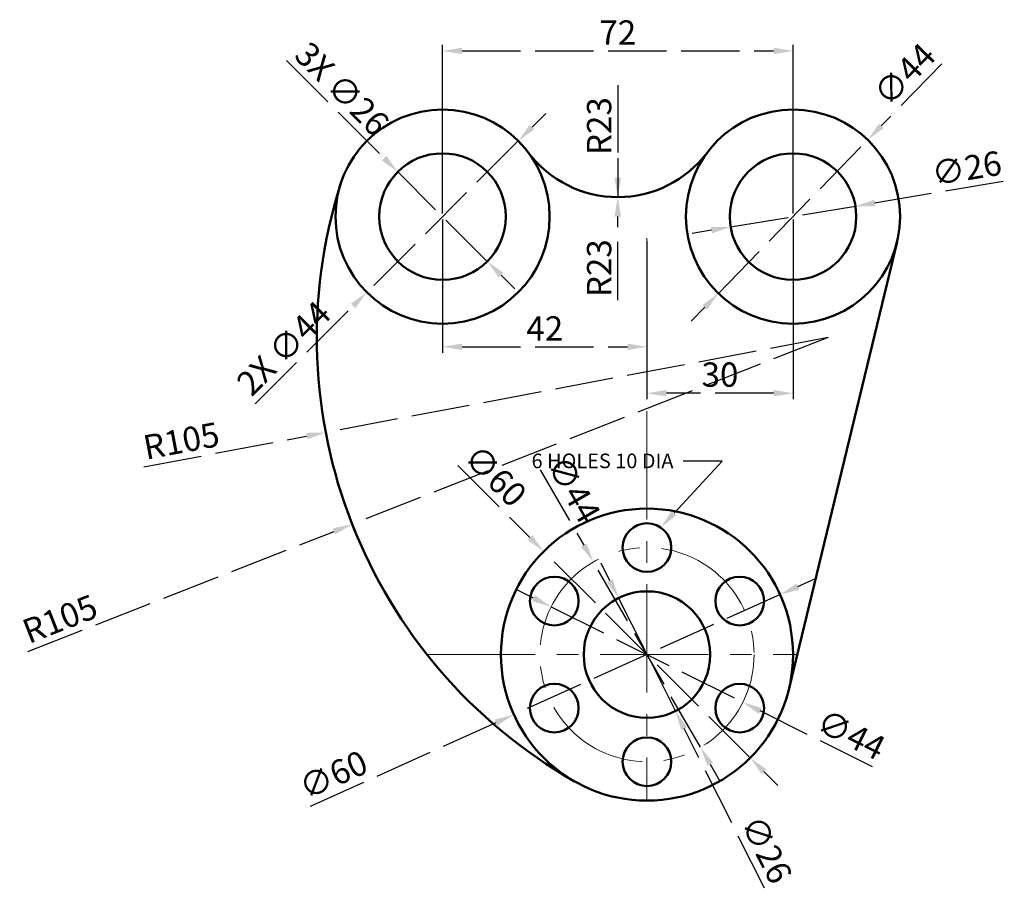
# Model space of a CAD drawing. Units: millimetres. Extents: x 2907 to 3109, y 1232 to 1411.
import ezdxf
from ezdxf import colors
from ezdxf.entities.mleader import LeaderData, LeaderLine
from ezdxf.math import Vec2, Vec3

# ---------------------------------------------------------------- set-up
doc = ezdxf.new("R2010")
doc.units = ezdxf.units.MM
doc.linetypes.add('ACAD_ISO02W100', pattern=[15, 12, -3])
doc.linetypes.add('CENTER', pattern=[50.8, 31.75, -6.35, 6.35, -6.35])
for name, color, linetype, lineweight in [('M-CNTR', 4, 'CENTER', 18), ('M-DIMS', 2, 'Continuous', 25), ('M-OUTL', 7, 'Continuous', 50), ('M-TEXT', 7, 'Continuous', 25)]:
    doc.layers.add(name, color=color, linetype=linetype, lineweight=lineweight)
doc.styles.get("Standard").update_dxf_attribs({"font": 'arial.ttf'})
doc.dimstyles.new('ISO-25', dxfattribs={"dimtxt": 5, "dimasz": 4, "dimexe": 1.25, "dimexo": 0.625, "dimtad": 1, "dimtxsty": 'Standard', "dimcen": 4, "dimadec": 0, "dimazin": 0, "dimtfac": 1, "dimtmove": 0, "dimatfit": 3, "dimfxl": 1, "dimlwd": -1, "dimarcsym": 0})

# ---------------------------------------------------------------- blocks, each defined once
blk = doc.blocks.new('*U1')
blk.add_circle((0, 0), 5)
blk = doc.blocks.new('*U2')
at = {"layer": 'M-OUTL', "color": 0, "linetype": 'ByBlock', "lineweight": -2, "transparency": 16777216}
blk.add_blockref('*U1', (3035.42, 1302.18), dxfattribs=at)
for p, rotation in [((3016.37, 1291.18), 59.99999999999999), ((3054.47, 1291.18), 300), ((3016.37, 1269.18), 120), ((3054.47, 1269.18), 240), ((3035.42, 1258.18), 180)]:
    blk.add_blockref('*U1', p, dxfattribs=dict(at, rotation=rotation))
blk = doc.blocks.new('*D3')
at = {"layer": 'Defpoints', "color": 0, "transparency": 16777216}
for p in [(3065.42, 1404.23), (2993.42, 1370.18), (3065.42, 1370.18)]:
    blk.add_point(p, dxfattribs=at)
at = {"layer": 'M-DIMS', "color": 0, "lineweight": -2, "transparency": 16777216}
for p, q in [((2993.42, 1370.81), (2993.42, 1405.48)), ((3065.42, 1370.81), (3065.42, 1405.48))]:
    blk.add_line(p, q, dxfattribs=at)
at = {"layer": 'M-DIMS', "color": 0, "linetype": 'ACAD_ISO02W100', "transparency": 16777216}
blk.add_line((2997.42, 1404.23), (3061.42, 1404.23), dxfattribs=at)
at = {"layer": 'M-DIMS', "color": 0, "transparency": 16777216}
for points in [[(2997.42, 1404.9), (2997.42, 1403.56), (2993.42, 1404.23)], [(3061.42, 1404.9), (3061.42, 1403.56), (3065.42, 1404.23)]]:
    blk.add_solid(points, dxfattribs=at)
at = {"layer": 'M-DIMS', "color": 0, "transparency": 16777216, "insert": (3029.42, 1407.36), "char_height": 5, "attachment_point": 5}
blk.add_mtext('72', dxfattribs=at)
blk = doc.blocks.new('*D4')
at = {"layer": 'Defpoints', "color": 0, "transparency": 16777216}
for p in [(3072.61, 1345.31), (2969.43, 1325.82)]:
    blk.add_point(p, dxfattribs=at)
at = {"layer": 'M-DIMS', "color": 0, "linetype": 'ACAD_ISO02W100', "transparency": 16777216}
for p, q in [((3072.61, 1345.31), (2969.43, 1325.82)), ((2932.05, 1318.76), (2965.5, 1325.08))]:
    blk.add_line(p, q, dxfattribs=at)
at = {"layer": 'M-DIMS', "color": 0, "transparency": 16777216}
blk.add_solid([(2965.38, 1325.74), (2965.63, 1324.43), (2969.43, 1325.82)], dxfattribs=at)
at = {"layer": 'M-DIMS', "color": 0, "transparency": 16777216, "insert": (2939.87, 1323.48), "char_height": 5, "attachment_point": 5, "rotation": 10.6961}
blk.add_mtext('R105', dxfattribs=at)
blk = doc.blocks.new('*D5')
at = {"layer": 'Defpoints', "color": 0, "transparency": 16777216}
for p in [(3029.42, 1397.18), (3029.42, 1374.18)]:
    blk.add_point(p, dxfattribs=at)
at = {"layer": 'M-DIMS', "color": 0, "linetype": 'ACAD_ISO02W100', "transparency": 16777216}
blk.add_line((3029.42, 1395.38), (3029.42, 1378.18), dxfattribs=at)
at = {"layer": 'M-DIMS', "color": 0, "transparency": 16777216}
blk.add_solid([(3028.75, 1378.18), (3030.09, 1378.18), (3029.42, 1374.18)], dxfattribs=at)
at = {"layer": 'M-DIMS', "color": 0, "transparency": 16777216, "insert": (3026.24, 1388.78), "char_height": 5, "attachment_point": 5, "rotation": 90}
blk.add_mtext('R23', dxfattribs=at)
blk = doc.blocks.new('*D6')
at = {"layer": 'Defpoints', "color": 0, "transparency": 16777216}
for p in [(3062.77, 1292.5), (3008.07, 1267.86)]:
    blk.add_point(p, dxfattribs=at)
at = {"layer": 'M-DIMS', "color": 0, "linetype": 'ACAD_ISO02W100', "transparency": 16777216}
for p, q in [((3066.42, 1294.15), (3070.07, 1295.79)), ((3062.77, 1292.5), (3008.07, 1267.86)), ((2966.29, 1249.04), (3004.42, 1266.22))]:
    blk.add_line(p, q, dxfattribs=at)
at = {"layer": 'M-DIMS', "color": 0, "transparency": 16777216}
for points in [[(3066.15, 1294.76), (3066.69, 1293.54), (3062.77, 1292.5)], [(3004.15, 1266.82), (3004.7, 1265.61), (3008.07, 1267.86)]]:
    blk.add_solid(points, dxfattribs=at)
at = {"layer": 'M-DIMS', "color": 0, "transparency": 16777216, "insert": (2971.24, 1254.9), "char_height": 5, "attachment_point": 5, "rotation": 24.2528}
blk.add_mtext('∅60', dxfattribs=at)
blk = doc.blocks.new('*D7')
at = {"layer": 'Defpoints', "color": 0, "transparency": 16777216}
for p in [(3015.72, 1289.98), (3055.12, 1270.38)]:
    blk.add_point(p, dxfattribs=at)
at = {"layer": 'M-DIMS', "color": 0, "linetype": 'ACAD_ISO02W100', "transparency": 16777216}
for p, q in [((3012.14, 1291.76), (3008.56, 1293.54)), ((3015.72, 1289.98), (3055.12, 1270.38)), ((3081.78, 1257.11), (3058.7, 1268.6))]:
    blk.add_line(p, q, dxfattribs=at)
at = {"layer": 'M-DIMS', "color": 0, "transparency": 16777216}
for points in [[(3012.44, 1292.36), (3011.85, 1291.17), (3015.72, 1289.98)], [(3059, 1269.2), (3058.4, 1268), (3055.12, 1270.38)]]:
    blk.add_solid(points, dxfattribs=at)
at = {"layer": 'M-DIMS', "color": 0, "transparency": 16777216, "insert": (3077.07, 1263.17), "char_height": 5, "attachment_point": 5, "rotation": 333.5478}
blk.add_mtext('∅44', dxfattribs=at)
blk = doc.blocks.new('*D8')
at = {"layer": 'Defpoints', "color": 0, "transparency": 16777216}
for p in [(3029.58, 1291.8), (3041.26, 1268.57)]:
    blk.add_point(p, dxfattribs=at)
at = {"layer": 'M-DIMS', "color": 0, "linetype": 'ACAD_ISO02W100', "transparency": 16777216}
for p, q in [((3027.78, 1295.37), (3025.99, 1298.94)), ((3029.58, 1291.8), (3041.26, 1268.57)), ((3059.56, 1232.18), (3043.06, 1264.99))]:
    blk.add_line(p, q, dxfattribs=at)
at = {"layer": 'M-DIMS', "color": 0, "transparency": 16777216}
for points in [[(3028.38, 1295.67), (3027.19, 1295.07), (3029.58, 1291.8)], [(3043.65, 1265.29), (3042.46, 1264.69), (3041.26, 1268.57)]]:
    blk.add_solid(points, dxfattribs=at)
at = {"layer": 'M-DIMS', "color": 0, "transparency": 16777216, "insert": (3059.41, 1239.85), "char_height": 5, "attachment_point": 5, "rotation": 296.6959}
blk.add_mtext('∅26', dxfattribs=at)
blk = doc.blocks.new('*D9')
at = {"layer": 'Defpoints', "color": 0, "transparency": 16777216}
for p in [(3080.76, 1385.95), (3050.08, 1354.41)]:
    blk.add_point(p, dxfattribs=at)
at = {"layer": 'M-DIMS', "color": 0, "linetype": 'ACAD_ISO02W100', "transparency": 16777216}
for p, q in [((3095.98, 1401.6), (3083.55, 1388.82)), ((3050.08, 1354.41), (3080.76, 1385.95)), ((3047.29, 1351.54), (3044.5, 1348.68))]:
    blk.add_line(p, q, dxfattribs=at)
at = {"layer": 'M-DIMS', "color": 0, "transparency": 16777216}
for points in [[(3083.07, 1389.28), (3084.03, 1388.35), (3080.76, 1385.95)], [(3046.82, 1352.01), (3047.77, 1351.08), (3050.08, 1354.41)]]:
    blk.add_solid(points, dxfattribs=at)
at = {"layer": 'M-DIMS', "color": 0, "transparency": 16777216, "insert": (3088.78, 1398.96), "char_height": 5, "attachment_point": 5, "rotation": 45.7945}
blk.add_mtext('∅44', dxfattribs=at)
blk = doc.blocks.new('*D10')
at = {"layer": 'Defpoints', "color": 0, "transparency": 16777216}
for p in [(3078.24, 1372.32), (3052.6, 1368.05)]:
    blk.add_point(p, dxfattribs=at)
at = {"layer": 'M-DIMS', "color": 0, "linetype": 'ACAD_ISO02W100', "transparency": 16777216}
for p, q in [((3108.57, 1377.37), (3082.19, 1372.97)), ((3052.6, 1368.05), (3078.24, 1372.32)), ((3048.65, 1367.39), (3044.71, 1366.73))]:
    blk.add_line(p, q, dxfattribs=at)
at = {"layer": 'M-DIMS', "color": 0, "transparency": 16777216}
for points in [[(3082.08, 1373.63), (3082.3, 1372.32), (3078.24, 1372.32)], [(3048.54, 1368.05), (3048.76, 1366.73), (3052.6, 1368.05)]]:
    blk.add_solid(points, dxfattribs=at)
at = {"layer": 'M-DIMS', "color": 0, "transparency": 16777216, "insert": (3101.19, 1379.5), "char_height": 5, "attachment_point": 5, "rotation": 9.4565}
blk.add_mtext('∅26', dxfattribs=at)
blk = doc.blocks.new('*D11')
at = {"layer": 'Defpoints', "color": 0, "transparency": 16777216}
for p in [(2993.42, 1370.18), (3035.42, 1365.74), (3035.42, 1343.43)]:
    blk.add_point(p, dxfattribs=at)
at = {"layer": 'M-DIMS', "color": 0, "lineweight": -2, "transparency": 16777216}
for p, q in [((2993.42, 1369.56), (2993.42, 1342.18)), ((3035.42, 1365.12), (3035.42, 1342.18))]:
    blk.add_line(p, q, dxfattribs=at)
at = {"layer": 'M-DIMS', "color": 0, "linetype": 'ACAD_ISO02W100', "transparency": 16777216}
blk.add_line((2997.42, 1343.43), (3031.42, 1343.43), dxfattribs=at)
at = {"layer": 'M-DIMS', "color": 0, "transparency": 16777216}
for points in [[(2997.42, 1344.09), (2997.42, 1342.76), (2993.42, 1343.43)], [(3031.42, 1344.09), (3031.42, 1342.76), (3035.42, 1343.43)]]:
    blk.add_solid(points, dxfattribs=at)
at = {"layer": 'M-DIMS', "color": 0, "transparency": 16777216, "insert": (3014.42, 1346.56), "char_height": 5, "attachment_point": 5}
blk.add_mtext('42', dxfattribs=at)
blk = doc.blocks.new('*D12')
at = {"layer": 'Defpoints', "color": 0, "transparency": 16777216}
for p in [(3065.42, 1370.18), (3035.42, 1364.89), (3035.42, 1333.89)]:
    blk.add_point(p, dxfattribs=at)
at = {"layer": 'M-DIMS', "color": 0, "lineweight": -2, "transparency": 16777216}
for p, q in [((3065.42, 1369.56), (3065.42, 1332.64)), ((3035.42, 1364.27), (3035.42, 1332.64))]:
    blk.add_line(p, q, dxfattribs=at)
at = {"layer": 'M-DIMS', "color": 0, "linetype": 'ACAD_ISO02W100', "transparency": 16777216}
blk.add_line((3061.42, 1333.89), (3039.42, 1333.89), dxfattribs=at)
at = {"layer": 'M-DIMS', "color": 0, "transparency": 16777216}
for points in [[(3039.42, 1334.56), (3039.42, 1333.23), (3035.42, 1333.89)], [(3061.42, 1334.56), (3061.42, 1333.23), (3065.42, 1333.89)]]:
    blk.add_solid(points, dxfattribs=at)
at = {"layer": 'M-DIMS', "color": 0, "transparency": 16777216, "insert": (3050.42, 1337.07), "char_height": 5, "attachment_point": 5}
blk.add_mtext('30', dxfattribs=at)
blk = doc.blocks.new('LUG-EYE-44-BORE-26')
for radius in [22, 13]:
    blk.add_circle((0, 0), radius)
blk = doc.blocks.new('*D14')
at = {"layer": 'Defpoints', "color": 0, "transparency": 16777216}
for p in [(3072.61, 1345.31), (2974.86, 1306.97)]:
    blk.add_point(p, dxfattribs=at)
at = {"layer": 'M-DIMS', "color": 0, "linetype": 'ACAD_ISO02W100', "transparency": 16777216}
for p, q in [((3072.61, 1345.31), (2974.86, 1306.97)), ((2908.24, 1280.83), (2971.14, 1305.51))]:
    blk.add_line(p, q, dxfattribs=at)
at = {"layer": 'M-DIMS', "color": 0, "transparency": 16777216}
blk.add_solid([(2970.89, 1306.13), (2971.38, 1304.88), (2974.86, 1306.97)], dxfattribs=at)
at = {"layer": 'M-DIMS', "color": 0, "transparency": 16777216, "insert": (2915.05, 1286.92), "char_height": 5, "attachment_point": 5, "rotation": 21.4205}
blk.add_mtext('R105', dxfattribs=at)
blk = doc.blocks.new('*D15')
at = {"layer": 'Defpoints', "color": 0, "transparency": 16777216}
for p in [(3029.42, 1397.18), (3029.42, 1374.18)]:
    blk.add_point(p, dxfattribs=at)
at = {"layer": 'M-DIMS', "color": 0, "linetype": 'ACAD_ISO02W100', "transparency": 16777216}
for p, q in [((3029.42, 1397.18), (3029.42, 1374.18)), ((3029.42, 1352.98), (3029.42, 1370.18))]:
    blk.add_line(p, q, dxfattribs=at)
at = {"layer": 'M-DIMS', "color": 0, "transparency": 16777216}
blk.add_solid([(3028.75, 1370.18), (3030.09, 1370.18), (3029.42, 1374.18)], dxfattribs=at)
at = {"layer": 'M-DIMS', "color": 0, "transparency": 16777216, "insert": (3026.24, 1359.58), "char_height": 5, "attachment_point": 5, "rotation": 89.9997}
blk.add_mtext('R23', dxfattribs=at)
blk = doc.blocks.new('*D16')
at = {"layer": 'Defpoints', "color": 0, "transparency": 16777216}
for p in [(2984.23, 1379.37), (3002.61, 1360.99)]:
    blk.add_point(p, dxfattribs=at)
at = {"layer": 'M-DIMS', "color": 0, "linetype": 'ACAD_ISO02W100', "transparency": 16777216}
for p, q in [((2961.37, 1402.23), (2981.4, 1382.2)), ((3002.61, 1360.99), (2984.23, 1379.37)), ((3005.44, 1358.16), (3008.27, 1355.33))]:
    blk.add_line(p, q, dxfattribs=at)
at = {"layer": 'M-DIMS', "color": 0, "transparency": 16777216}
for points in [[(2981.87, 1382.67), (2980.93, 1381.73), (2984.23, 1379.37)], [(3005.91, 1358.63), (3004.97, 1357.69), (3002.61, 1360.99)]]:
    blk.add_solid(points, dxfattribs=at)
at = {"layer": 'M-DIMS', "color": 0, "transparency": 16777216, "insert": (2972.32, 1395.98), "char_height": 5, "attachment_point": 5, "rotation": 315.0016}
blk.add_mtext('3X ∅26', dxfattribs=at)
blk = doc.blocks.new('*D17')
at = {"layer": 'Defpoints', "color": 0, "transparency": 16777216}
for p in [(3008.98, 1385.74), (2977.86, 1354.62)]:
    blk.add_point(p, dxfattribs=at)
at = {"layer": 'M-DIMS', "color": 0, "linetype": 'ACAD_ISO02W100', "transparency": 16777216}
for p, q in [((3011.81, 1388.57), (3014.63, 1391.39)), ((3008.98, 1385.74), (2977.86, 1354.62)), ((2954.96, 1331.72), (2975.04, 1351.8))]:
    blk.add_line(p, q, dxfattribs=at)
at = {"layer": 'M-DIMS', "color": 0, "transparency": 16777216}
for points in [[(3011.33, 1389.04), (3012.28, 1388.09), (3008.98, 1385.74)], [(2974.57, 1352.27), (2975.51, 1351.33), (2977.86, 1354.62)]]:
    blk.add_solid(points, dxfattribs=at)
at = {"layer": 'M-DIMS', "color": 0, "transparency": 16777216, "insert": (2961.24, 1342.69), "char_height": 5, "attachment_point": 5, "rotation": 45.0004}
blk.add_mtext('2X ∅44', dxfattribs=at)
blk = doc.blocks.new('*D18')
at = {"layer": 'Defpoints', "color": 0, "transparency": 16777216}
for p in [(3024.42, 1299.23), (3046.42, 1261.13)]:
    blk.add_point(p, dxfattribs=at)
at = {"layer": 'M-DIMS', "color": 0, "linetype": 'ACAD_ISO02W100', "transparency": 16777216}
for p, q in [((3013.5, 1318.14), (3022.42, 1302.7)), ((3046.42, 1261.13), (3024.42, 1299.23)), ((3048.42, 1257.67), (3050.42, 1254.2))]:
    blk.add_line(p, q, dxfattribs=at)
at = {"layer": 'M-DIMS', "color": 0, "transparency": 16777216}
for points in [[(3023, 1303.03), (3021.84, 1302.36), (3024.42, 1299.23)], [(3049, 1258), (3047.84, 1257.33), (3046.42, 1261.13)]]:
    blk.add_solid(points, dxfattribs=at)
at = {"layer": 'M-DIMS', "color": 0, "transparency": 16777216, "insert": (3019.84, 1313.81), "char_height": 5, "attachment_point": 5, "rotation": 300.0015}
blk.add_mtext('∅44', dxfattribs=at)
blk = doc.blocks.new('*D19')
at = {"layer": 'Defpoints', "color": 0, "transparency": 16777216}
for p in [(3014.21, 1301.39), (3056.63, 1258.97)]:
    blk.add_point(p, dxfattribs=at)
at = {"layer": 'M-DIMS', "color": 0, "linetype": 'ACAD_ISO02W100', "transparency": 16777216}
for p, q in [((2996.59, 1319.01), (3011.38, 1304.22)), ((3056.63, 1258.97), (3014.21, 1301.39)), ((3059.46, 1256.14), (3062.29, 1253.31))]:
    blk.add_line(p, q, dxfattribs=at)
at = {"layer": 'M-DIMS', "color": 0, "transparency": 16777216}
for points in [[(3011.85, 1304.69), (3010.91, 1303.75), (3014.21, 1301.39)], [(3059.93, 1256.61), (3058.99, 1255.67), (3056.63, 1258.97)]]:
    blk.add_solid(points, dxfattribs=at)
at = {"layer": 'M-DIMS', "color": 0, "transparency": 16777216, "insert": (3003.83, 1316.47), "char_height": 5, "attachment_point": 5, "rotation": 315.0007}
blk.add_mtext('∅60', dxfattribs=at)

msp = doc.modelspace()

# ---------------------------------------------------------------- linework, layer by layer
at = {"layer": 'M-CNTR', "ltscale": 0.7}
for p, q in [((3035.421, 1365.745), (3035.421, 1250.181)), ((2990.25, 1280.181), (3066.286, 1280.181))]:
    msp.add_line(p, q, dxfattribs=at)
msp.add_circle((3035.421, 1280.181), 22, dxfattribs=at)
at = {"layer": 'M-OUTL'}
msp.add_line((3064.623, 1273.309), (3086.804, 1365.009), dxfattribs=at)
for radius in [30, 13]:
    msp.add_circle((3035.421, 1280.181), radius, dxfattribs=at)
for centre, radius, start, end in [((3029.421, 1397.181), 23, 216.8699, 323.1301), ((3072.608, 1345.313), 105, 162.56531, 240.27581)]:
    msp.add_arc(centre, radius, start, end, dxfattribs=at)

# ---------------------------------------------------------------- block references
for name, p in [('LUG-EYE-44-BORE-26', (2993.421, 1370.181)), ('LUG-EYE-44-BORE-26', (3065.421, 1370.181)), ('*U2', (0, 0))]:
    msp.add_blockref(name, p, dxfattribs=at)

# ---------------------------------------------------------------- dimensions: what is measured, and where the dimension line sits
at = {"layer": 'M-DIMS'}
for base, p1, p2, picture, middle in [((3065.421, 1404.23), (2993.421, 1370.181), (3065.421, 1370.181), '*D3', (3029.421, 1407.365)), ((3035.421, 1343.427), (2993.421, 1370.181), (3035.421, 1365.745), '*D11', (3014.421, 1346.563)), ((3035.421, 1333.895), (3065.421, 1370.181), (3035.421, 1364.892), '*D12', (3050.421, 1337.074))]:
    dim = msp.add_linear_dim(base=base, p1=p1, p2=p2, dimstyle='ISO-25', override={"dimclrd": 0, "dimclre": 0, "dimclrt": 0}, dxfattribs=at)
    dim.commit()
    dim.dimension.update_dxf_attribs({"geometry": picture, "text_midpoint": middle})
for p1, p2, text, picture, middle in [((3002.614, 1360.989), (2984.229, 1379.373), '3X <>', '*D16', (2969.972, 1393.629)), ((3008.977, 1385.738), (2977.865, 1354.625), '2X <>', '*D17', (2963.583, 1340.343))]:
    dim = msp.add_diameter_dim_2p(p1=p1, p2=p2, text=text, dimstyle='ISO-25', override={"dimdec": 0, "dimlfac": 1, "dimrnd": 0, "dimzin": 0, "dimdsep": 46, "dimlunit": 2}, dxfattribs=at)
    dim.commit()
    dim.dimension.update_dxf_attribs({"geometry": picture, "text_midpoint": middle})
for p1, p2, override, picture, middle in [((3050.082, 1354.411), (3080.76, 1385.952), {"dimclrd": 0, "dimclre": 0, "dimclrt": 0}, '*D9', (3088.782, 1398.958)), ((3046.422, 1261.129), (3024.421, 1299.234), {"dimdec": 0, "dimlfac": 1, "dimrnd": 0, "dimzin": 0, "dimdsep": 46, "dimlunit": 2}, '*D18', (3016.962, 1312.151))]:
    dim = msp.add_diameter_dim_2p(p1=p1, p2=p2, dimstyle='ISO-25', override=override, dxfattribs=at)
    dim.commit()
    dim.dimension.update_dxf_attribs({"geometry": picture, "text_midpoint": middle})
dim = msp.add_radius_dim(center=(3029.421, 1397.181), mpoint=(3029.421, 1374.181), dimstyle='ISO-25', override={"dimdec": 0, "dimlfac": 1, "dimrnd": 0, "dimzin": 0, "dimdsep": 46, "dimlunit": 2}, dxfattribs=at)
dim.commit()
dim.dimension.update_dxf_attribs({"geometry": '*D15', "text_midpoint": (3026.241, 1359.583)})
for center, mpoint, override, picture, middle in [((3029.421, 1397.181), (3029.421, 1374.181), {"dimclrd": 0, "dimclre": 0, "dimclrt": 0}, '*D5', (3029.421, 1388.78)), ((3072.608, 1345.313), (2974.861, 1306.966), {"dimdec": 0, "dimlfac": 1, "dimrnd": 0, "dimzin": 0, "dimdsep": 46, "dimlunit": 2}, '*D14', (2916.213, 1283.958)), ((3072.608, 1345.313), (2969.432, 1325.825), {"dimclrd": 0, "dimclre": 0, "dimclrt": 0}, '*D4', (2940.462, 1320.353))]:
    dim = msp.add_radius_dim(center=center, mpoint=mpoint, dimstyle='ISO-25', override=override, dxfattribs=at)
    dim.commit()
    dim.dimension.update_dxf_attribs({"geometry": picture, "text_midpoint": middle, "dimtype": 164})
for p1, p2, override, picture, middle in [((3052.598, 1368.045), (3078.244, 1372.317), {"dimclrd": 0, "dimclre": 0, "dimclrt": 0}, '*D10', (3101.737, 1376.23)), ((3056.635, 1258.968), (3014.208, 1301.394), {"dimdec": 0, "dimlfac": 1, "dimrnd": 0, "dimzin": 0, "dimdsep": 46, "dimlunit": 2}, '*D19', (3001.48, 1314.122)), ((3029.581, 1291.796), (3041.261, 1268.567), {"dimclrd": 0, "dimclre": 0, "dimclrt": 0}, '*D8', (3056.449, 1238.364)), ((3062.773, 1292.504), (3008.069, 1267.858), {"dimclrd": 0, "dimclre": 0, "dimclrt": 0}, '*D6', (2972.6, 1251.879)), ((3015.724, 1289.981), (3055.118, 1270.381), {"dimclrd": 0, "dimclre": 0, "dimclrt": 0}, '*D7', (3075.591, 1260.195))]:
    dim = msp.add_diameter_dim_2p(p1=p1, p2=p2, dimstyle='ISO-25', override=override, dxfattribs=at)
    dim.commit()
    dim.dimension.update_dxf_attribs({"geometry": picture, "text_midpoint": middle, "dimtype": 163})

# ---------------------------------------------------------------- leaders
at = {"layer": 'M-TEXT'}
ml = msp.add_multileader_mtext('Standard', dxfattribs=at)
ml.set_content('6 HOLES 10 DIA', color=256)
ml.set_leader_properties()
ml.build(insert=Vec2(0, 0))
ctx = ml.context
ctx.base_point, ctx.char_height, ctx.plane_origin = Vec3(3007.335, 1319.962), 3, Vec3(3038.26, 1306.297)
ctx.text_align_type = 2
notes = []
notes.append((ctx, [(0, (1, 1, 0), (3050.864, 1319.962), (-1, 0), 8, [(0, [(3038.26, 1306.297)], 0, [])])]))
ctx.mtext.insert, ctx.mtext.alignment, ctx.mtext.flow_direction = Vec3(3040.864, 1321.488), 3, 5
for ctx, leaders in notes:
    for number, flags, end, landing, length, lines in leaders:
        leader = LeaderData()
        leader.index, (leader.has_last_leader_line, leader.has_dogleg_vector, leader.attachment_direction) = number, flags
        leader.last_leader_point, leader.dogleg_vector, leader.dogleg_length = Vec3(end), Vec3(landing), length
        for number, points, colour, breaks in lines:
            line = LeaderLine()
            line.index, line.vertices, line.color, line.breaks = number, Vec3.list(points), colors.encode_raw_color(colour), breaks
            leader.lines.append(line)
        ctx.leaders.append(leader)

doc.saveas('drawing.dxf')
